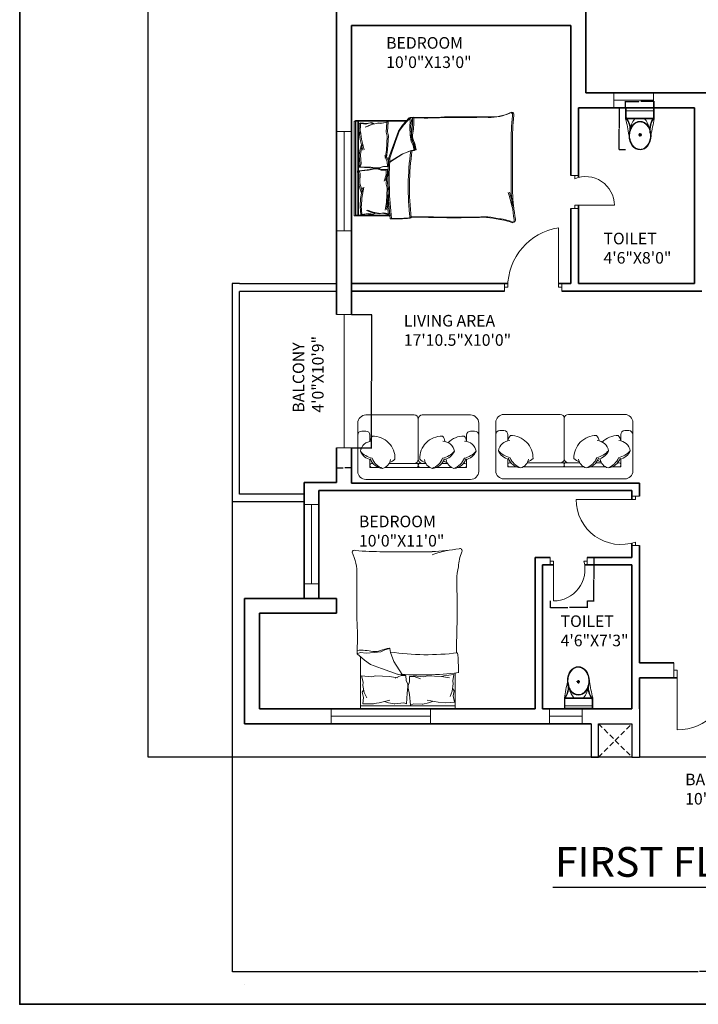
# Model space of a CAD drawing. Units: inches. Extents: x 2296 to 3812, y -1531 to 2564.
# Tile 1 of 10: x 2296 to 2706, y 1124 to 1719. Entities that reach past the tile are written whole.
import ezdxf

# ---------------------------------------------------------------- set-up
doc = ezdxf.new("R2010")
doc.units = ezdxf.units.IN
doc.linetypes.add('HIDDEN2', pattern=[4.7625, 3.175, -1.5875])
for name, color, linetype, lineweight in [('A-ANNO-DIMS', 2, 'Continuous', 18), ('A-ANNO-TEXT', 7, 'Continuous', 25), ('A-ANNO-TTLB', 7, 'Continuous', 35), ('A-AREA-IDEN', 7, 'Continuous', 18), ('A-DOOR', 3, 'Continuous', 18), ('A-FLOR-FIXT', 9, 'Continuous', 18), ('A-FLOR-HRAL', 7, 'Continuous', 25), ('A-FURN', 8, 'Continuous', 18), ('A-GLAZ', 4, 'Continuous', 18), ('A-REF', 8, 'Continuous', 13), ('A-WALL', 7, 'Continuous', 35), ('A-WALL-HIDN', 8, 'HIDDEN2', 18)]:
    doc.layers.add(name, color=color, linetype=linetype, lineweight=lineweight)
doc.styles.get("Standard").update_dxf_attribs({"font": 'arial.ttf'})
doc.dimstyles.get("Standard").update_dxf_attribs({"dimtxt": 0.18, "dimasz": 0.18, "dimexe": 0.18, "dimexo": 0.0625, "dimgap": 0.09, "dimtad": 0, "dimtih": 1, "dimtoh": 1, "dimdec": 4, "dimzin": 0, "dimdsep": 46, "dimtxsty": 'Standard', "dimcen": 0.09, "dimadec": 0, "dimazin": 0, "dimtfac": 1, "dimtdec": 4, "dimtofl": 0, "dimtmove": 0, "dimatfit": 3, "dimfxl": 1, "dimtolj": 1, "dimtzin": 0, "dimarcsym": 0})

# ---------------------------------------------------------------- blocks, each defined once
blk = doc.blocks.new('A$C31115884')
for p, q in [((283, 498), (223, 498)), ((258, 466), (258, 523)), ((0, 200), (0, 0)), ((520, 200), (0, 200)), ((10, 190), (10, 10)), ((510, 190), (10, 190)), ((510, 10), (510, 190)), ((520, 0), (520, 200)), ((510, 54), (0, 54)), ((10, 10), (510, 10)), ((0, 0), (520, 0))]:
    blk.add_line(p, q)
blk.add_circle((256, 496), 23.6)
for centre, radius, start, end in [((2778, -205), 2807, 165.4549, 171.7133), ((-295, 403), 365, 324.2091, 9.3499), ((-295, 403), 375, 324.2091, 9.3499), ((139, 406), 293, 315.8436, 2.6563), ((806, 403), 375, 179.2036, 215.7909), ((806, 403), 365, 170.6501, 215.7909), ((3237, 905), 2807, 188.2867, 194.5451), ((384, 406), 293, 190.2774, 224.1564)]:
    blk.add_arc(centre, radius, start, end)
blk.add_ellipse((256, 510), major_axis=(0, -261), ratio=0.772727)
blk.add_open_spline([(256, 259), (263, 259), (270, 260), (288, 262), (299, 265), (320, 273), (330, 278), (350, 291), (360, 299), (378, 316), (386, 326), (402, 347), (409, 358), (421, 383), (427, 395), (436, 422), (440, 436), (445, 465), (447, 480), (448, 509), (448, 524), (445, 553), (443, 568), (436, 596), (432, 610), (422, 636), (416, 649), (402, 672), (395, 683), (379, 703), (370, 712), (351, 728), (341, 735), (321, 746), (310, 751), (289, 757), (278, 759), (256, 761), (245, 761), (223, 757), (212, 754), (191, 746), (181, 741), (161, 728), (151, 720), (133, 703), (125, 693), (110, 672), (103, 660), (90, 636), (85, 623), (76, 596), (72, 582), (67, 553), (66, 538), (64, 509), (65, 494), (68, 465), (70, 450), (77, 422), (81, 408), (91, 382), (97, 370), (111, 346), (118, 335), (135, 316), (144, 307), (162, 291), (172, 284), (193, 273), (203, 269), (225, 262), (236, 260), (250, 259), (253, 259), (256, 259)], degree=3, knots=[0, 0, 0, 0, 0.110105, 0.110105, 0.285049, 0.285049, 0.459994, 0.459994, 0.634938, 0.634938, 0.809882, 0.809882, 0.984827, 0.984827, 1.159771, 1.159771, 1.334715, 1.334715, 1.50966, 1.50966, 1.684604, 1.684604, 1.859549, 1.859549, 2.034493, 2.034493, 2.209437, 2.209437, 2.384382, 2.384382, 2.559326, 2.559326, 2.73427, 2.73427, 2.909215, 2.909215, 3.084159, 3.084159, 3.259103, 3.259103, 3.434048, 3.434048, 3.608992, 3.608992, 3.783936, 3.783936, 3.958881, 3.958881, 4.133825, 4.133825, 4.30877, 4.30877, 4.483714, 4.483714, 4.658658, 4.658658, 4.833603, 4.833603, 5.008547, 5.008547, 5.183491, 5.183491, 5.358436, 5.358436, 5.53338, 5.53338, 5.708324, 5.708324, 5.883269, 5.883269, 6.058213, 6.058213, 6.233158, 6.233158, 6.283185, 6.283185, 6.283185, 6.283185])
blk = doc.blocks.new('DOOR-BEDROOM-36-WS')
for p, q in [((32.71, 2.25), (32.71, 38.25)), ((0, 4.5), (0, 0)), ((0, 0), (0, 2.25)), ((0, 2.25), (2, 2.25)), ((34.71, 2.25), (32.71, 2.25)), ((34.71, 4.5), (34.71, 0)), ((34.71, 0), (34.71, 2.25))]:
    blk.add_line(p, q)
blk.add_arc((38.45, 2.25), 36.46, 99.06194, 180)
blk = doc.blocks.new('DOOR-BATH-24-SW')
for p, q in [((0, 26.25), (0, 21.75)), ((0, 21.75), (0, 24)), ((0, 24), (2, 24)), ((2, 24), (2, 0)), ((22.44, 24), (20.44, 24)), ((22.44, 26.25), (22.44, 21.75)), ((22.44, 21.75), (22.44, 24))]:
    blk.add_line(p, q)
blk.add_arc((2, 19.08), 19.08, 270, 14.93359)
blk = doc.blocks.new('DOOR-BEDROOM-36-SW')
for p, q in [((36, 27.71), (0, 27.71)), ((38.25, 29.71), (33.75, 29.71)), ((33.75, 29.71), (36, 29.71)), ((36, 29.71), (36, 27.71)), ((36, 0), (36, 2)), ((33.75, 0), (38.25, 0)), ((38.25, 0), (36, 0))]:
    blk.add_line(p, q)
blk.add_arc((27.18, 27.71), 27.18, 180, 288.93127)
blk = doc.blocks.new('DOOR-BALCONY-PAIR-S')
for p, q in [((0, 40.5), (0, 31.5)), ((0, 31.5), (0, 36)), ((0, 36), (2, 36)), ((2, 36), (2, 0)), ((65.68, 36), (63.68, 36)), ((63.68, 36), (63.68, 0)), ((65.68, 40.5), (65.68, 31.5)), ((65.68, 31.5), (65.68, 36))]:
    blk.add_line(p, q)
for centre, radius, start, end in [((2, 31.87), 31.87, 270, 359.32793), ((65.8, 31.86), 31.93, 180.64039, 266.18908)]:
    blk.add_arc(centre, radius, start, end)
blk = doc.blocks.new('DOOR-BATH-24-WS')
for p, q in [((0, 20), (4.5, 20)), ((4.5, 20), (2.25, 20)), ((2.25, 20), (2.25, 18)), ((2.25, 0), (2.25, 2)), ((2.25, 2), (26.25, 2)), ((0, 0), (4.5, 0)), ((4.5, 0), (2.25, 0))]:
    blk.add_line(p, q)
blk.add_arc((8.92, 2), 17.33, 0, 112.62699)
blk = doc.blocks.new('WIN-60-JAMB-A')
for p, q in [((0, 60), (9, 60)), ((9, 60), (4.5, 60)), ((4.5, 60), (4.5, 0)), ((9, 0), (0, 0)), ((4.5, 0), (9, 0))]:
    blk.add_line(p, q)
blk = doc.blocks.new('WIN-48-BEDROOM-SW')
for p, q in [((0, 48), (9, 48)), ((9, 48), (4.5, 48)), ((4.5, 48), (4.5, 0)), ((9, 0), (0, 0)), ((4.5, 0), (9, 0))]:
    blk.add_line(p, q)
blk = doc.blocks.new('WIN-24-SHAFT-S')
for p, q in [((0, 9), (0, 0)), ((24, 4.5), (24, 9)), ((24, 9), (24, 0)), ((0, 0), (0, 4.5)), ((0, 4.5), (0, 4.5)), ((0, 4.5), (24, 4.5))]:
    blk.add_line(p, q)
blk = doc.blocks.new('WIN-60-SILL')
for p, q in [((0, 9), (0, 0)), ((60, 4.5), (60, 9)), ((60, 9), (60, 0)), ((0, 0), (0, 4.5)), ((0, 4.5), (60, 4.5))]:
    blk.add_line(p, q)
blk = doc.blocks.new('WIN-20-VENT')
for p, q in [((0, 9), (0, 0)), ((19.57, 4.5), (19.57, 9)), ((19.57, 9), (19.57, 0)), ((0, 0), (0, 4.5)), ((0, 4.5), (0, 4.5)), ((0, 4.5), (19.57, 4.5)), ((19.57, 0), (19.57, 0))]:
    blk.add_line(p, q)
blk = doc.blocks.new('GLAZ-BALCONY-S')
for p, q in [((0, 80.52), (9, 80.52)), ((4.5, 80.52), (4.5, 0)), ((0, 0), (9, 0))]:
    blk.add_line(p, q)
blk = doc.blocks.new('BED-DOUBLE')
for p, q in [((48.49, 95), (18.98, 95)), ((22.83, 36.42), (19.86, 35.68)), ((23.21, 34.01), (22.83, 36.42)), ((3.07, 35.36), (3.17, 33.26, 4.64)), ((5.01, 34.01), (3.17, 33.26)), ((3.17, 33.26), (7.61, 29.37)), ((8.72, 33.63), (5.01, 34.01)), ((5.09, 0), (5.09, 31.9)), ((13.37, 34.01), (8.72, 33.63)), ((17.45, 34.56), (13.37, 34.01)), ((19.86, 35.68), (17.45, 34.56)), ((25.25, 28.62), (23.21, 34.01)), ((7.61, 29.37), (11.14, 26.77)), ((11.14, 26.77), (17.82, 24.36)), ((17.82, 24.36), (27.82, 20.84)), ((30.27, 20.84), (25.25, 28.62)), ((11.92, 19.38), (5.77, 19.87)), ((5.77, 19.87), (6.7, 16.11)), ((14.27, 20.05), (11.92, 19.38)), ((22.67, 19.54), (14.27, 20.05)), ((27.51, 18.74), (22.67, 19.54)), ((29.68, 20.07), (26, 18.53)), ((32.62, 20.25), (29.68, 20.07)), ((32.82, 17.04), (32.62, 20.25)), ((34.71, 16.28), (34.71, 19.5)), ((34.71, 19.5), (37.65, 19.5)), ((43.31, 19.38), (37.16, 19.87)), ((37.65, 19.5), (41.42, 18.19)), ((45.66, 20.05), (43.31, 19.38)), ((54.06, 19.54), (45.66, 20.05)), ((54.06, 19.54), (55.42, 19.92)), ((58.9, 18.74), (54.06, 19.54)), ((55.42, 19.92), (61.53, 20.79)), ((61.53, 20.79), (60.84, 16.98)), ((62.38, 21.71), (62.38, 0)), ((6.7, 16.11), (6.47, 14.18)), ((6.47, 14.18), (7.43, 9.9)), ((33.66, 14.84), (32.82, 17.04)), ((33.3, 9.43), (33.75, 13.28)), ((33.75, 13.28), (33.66, 14.84)), ((34.01, 14.03), (34.71, 16.28)), ((34.01, 12.47), (34.01, 14.03)), ((34.71, 8.66), (34.01, 12.47)), ((61.19, 15.07), (60.49, 10.74)), ((60.84, 16.98), (61.19, 15.07)), ((61.71, 10.91), (61.01, 12.12)), ((6.21, 10), (6.83, 11.25)), ((6.93, 6.92), (6.21, 10)), ((6.47, 3.07), (6.93, 6.92)), ((7.43, 9.9), (8.85, 6.69)), ((33.01, 2.99), (33.3, 9.43)), ((35.4, 2.24), (34.71, 8.66)), ((60.49, 10.74), (59.28, 7.44)), ((61.19, 7.79), (61.71, 10.91)), ((61.88, 3.98), (61.19, 7.79)), ((62.38, 1.84), (5.09, 1.84)), ((62.38, 0), (5.09, 0)), ((6.47, 3.07), (12.95, 2.95)), ((11.75, 3.05), (16.3, 3.68)), ((12.95, 2.95), (11.75, 3.05)), ((16.3, 3.68), (22.8, 5.3)), ((19.55, 4.4), (22.03, 3.69)), ((22.03, 3.69), (25.54, 3.04)), ((25.54, 3.04), (25.93, 3.07)), ((25.93, 3.07), (31.24, 3.57)), ((31.24, 3.57), (33.01, 2.99)), ((37.13, 2.94), (35.4, 2.24)), ((42.46, 2.76), (37.13, 2.94)), ((42.85, 2.76), (42.46, 2.76)), ((46.31, 3.63), (42.85, 2.76)), ((52.03, 3.98), (45.45, 5.19)), ((48.74, 4.5), (46.31, 3.63)), ((56.62, 3.63), (52.03, 3.98)), ((56.74, 3.61), (56.62, 3.63)), ((61.87, 4), (56.74, 3.61))]:
    blk.add_line(p, q)
for centre, radius, start, end in [((1.32, 94.55), 1.32, 62.65876, 176.02002), ((17.21, 254.49), 159.5, 264.4998, 270.63509), ((87.19, -28.43), 127.63, 103.38322, 107.70533), ((40.86, 240.78), 145.97, 272.99578, 279.40907), ((65.24, 95.57), 1.31, 326.17358, 113.47814), ((-24.75, 82.32), 27.65, 357.47136, 26.46809), ((92.52, 84.25), 28.25, 157.97508, 176.652), ((98.8, 77.34), 35.53, 166.06484, 178.91125), ((5471.89, 81.31), 5469.02, 180.00217, 180.28689), ((-514.68, 60.68), 578.22, 358.22771, 1.71854), ((-151.96, 43.54), 155.25, 356.97912, 3.83645), ((267.13, 37.37), 203.94, 178.4762, 181.00819), ((29.2, 1.78), 35.55, 100.66171, 109.88058), ((22.63, 36.49), 0.221, 340.24637, 91.13765), ((5.01, -7.98), 43.38, 79.87628, 92.56571), ((14.11, 42.04), 7.46, 258.6608, 293.73842), ((45.26, 187.4), 154.68, 261.78449, 276.90062), ((-35.55, 24.09), 99.87, 358.72178, 5.60397), ((40.94, 218.26), 197.77, 266.08655, 276.78213)]:
    blk.add_arc(centre, radius, start, end)
blk = doc.blocks.new('*D45')
at = {"layer": 'A-ANNO-DIMS', "color": 0, "lineweight": -2, "transparency": 16777216}
for p, q in [((2662.39, 1665.95), (2658.45, 1665.95)), ((2658.63, 1665.77), (2658.63, 1653.39)), ((2658.63, 1640.65), (2658.63, 1653.03)), ((2662.39, 1640.47), (2658.45, 1640.47))]:
    blk.add_line(p, q, dxfattribs=at)
at = {"layer": 'A-ANNO-DIMS', "color": 0, "transparency": 16777216}
for points in [[(2658.6, 1665.77), (2658.66, 1665.77), (2658.63, 1665.95)], [(2658.6, 1640.65), (2658.66, 1640.65), (2658.63, 1640.47)]]:
    blk.add_solid(points, dxfattribs=at)
at = {"layer": 'Defpoints', "color": 0, "transparency": 16777216}
for p in [(2662.45, 1665.95), (2658.63, 1640.47), (2662.45, 1640.47)]:
    blk.add_point(p, dxfattribs=at)
at = {"layer": 'A-ANNO-DIMS', "color": 0, "transparency": 16777216, "insert": (2658.63, 1653.21), "char_height": 0.18, "attachment_point": 5}
blk.add_mtext('\\A1;WC 25 TYP.', dxfattribs=at)
blk = doc.blocks.new('*D46')
at = {"layer": 'A-ANNO-DIMS', "color": 0, "lineweight": -2, "transparency": 16777216}
for p, q in [((2662.45, 1666.01), (2662.45, 1669.95)), ((2662.63, 1669.77), (2670.53, 1669.77)), ((2679.46, 1669.77), (2671.57, 1669.77)), ((2679.64, 1666.01), (2679.64, 1669.95))]:
    blk.add_line(p, q, dxfattribs=at)
at = {"layer": 'A-ANNO-DIMS', "color": 0, "transparency": 16777216}
for points in [[(2662.63, 1669.8), (2662.63, 1669.74), (2662.45, 1669.77)], [(2679.46, 1669.8), (2679.46, 1669.74), (2679.64, 1669.77)]]:
    blk.add_solid(points, dxfattribs=at)
at = {"layer": 'Defpoints', "color": 0, "transparency": 16777216}
for p in [(2662.45, 1669.77), (2662.45, 1665.95), (2679.64, 1665.95)]:
    blk.add_point(p, dxfattribs=at)
at = {"layer": 'A-ANNO-DIMS', "color": 0, "transparency": 16777216, "insert": (2671.05, 1669.77), "char_height": 0.18, "attachment_point": 5}
blk.add_mtext('\\A1;17 TYP.', dxfattribs=at)
blk = doc.blocks.new('*D83')
at = {"layer": 'A-ANNO-DIMS', "color": 0, "lineweight": -2, "transparency": 16777216}
for p, q in [((2639.31, 1394.1), (2643.37, 1394.1)), ((2643.19, 1393.92), (2643.19, 1381.16)), ((2643.19, 1368.03), (2643.19, 1380.79)), ((2639.31, 1367.85), (2643.37, 1367.85))]:
    blk.add_line(p, q, dxfattribs=at)
at = {"layer": 'A-ANNO-DIMS', "color": 0, "transparency": 16777216}
for points in [[(2643.16, 1393.92), (2643.22, 1393.92), (2643.19, 1394.1)], [(2643.16, 1368.03), (2643.22, 1368.03), (2643.19, 1367.85)]]:
    blk.add_solid(points, dxfattribs=at)
at = {"layer": 'Defpoints', "color": 0, "transparency": 16777216}
for p in [(2639.25, 1394.1), (2643.19, 1394.1), (2639.25, 1367.85)]:
    blk.add_point(p, dxfattribs=at)
at = {"layer": 'A-ANNO-DIMS', "color": 0, "transparency": 16777216, "insert": (2643.19, 1380.98), "char_height": 0.18, "attachment_point": 5}
blk.add_mtext('\\A1;BATH DOOR 26 TYP.', dxfattribs=at)
blk = doc.blocks.new('*D84')
at = {"layer": 'A-ANNO-DIMS', "color": 0, "lineweight": -2, "transparency": 16777216}
for p, q in [((2616.81, 1367.79), (2616.81, 1363.73)), ((2616.99, 1363.91), (2627.5, 1363.91)), ((2639.07, 1363.91), (2628.56, 1363.91)), ((2639.25, 1367.79), (2639.25, 1363.73))]:
    blk.add_line(p, q, dxfattribs=at)
at = {"layer": 'A-ANNO-DIMS', "color": 0, "transparency": 16777216}
for points in [[(2616.99, 1363.94), (2616.99, 1363.88), (2616.81, 1363.91)], [(2639.07, 1363.94), (2639.07, 1363.88), (2639.25, 1363.91)]]:
    blk.add_solid(points, dxfattribs=at)
at = {"layer": 'Defpoints', "color": 0, "transparency": 16777216}
for p in [(2616.81, 1367.85), (2639.25, 1367.85), (2639.25, 1363.91)]:
    blk.add_point(p, dxfattribs=at)
at = {"layer": 'A-ANNO-DIMS', "color": 0, "transparency": 16777216, "insert": (2628.03, 1363.91), "char_height": 0.18, "attachment_point": 5}
blk.add_mtext('\\A1;22 TYP.', dxfattribs=at)
blk = doc.blocks.new('*D123')
at = {"layer": 'A-ANNO-DIMS', "color": 0, "lineweight": -2, "transparency": 16777216}
for p, q in [((2496.81, 1540.93), (2509.01, 1540.93)), ((2508.83, 1540.75), (2508.83, 1500.85)), ((2508.83, 1460.59), (2508.83, 1500.49)), ((2496.81, 1460.41), (2509.01, 1460.41))]:
    blk.add_line(p, q, dxfattribs=at)
at = {"layer": 'A-ANNO-DIMS', "color": 0, "transparency": 16777216}
for points in [[(2508.8, 1540.75), (2508.86, 1540.75), (2508.83, 1540.93)], [(2508.8, 1460.59), (2508.86, 1460.59), (2508.83, 1460.41)]]:
    blk.add_solid(points, dxfattribs=at)
at = {"layer": 'Defpoints', "color": 0, "transparency": 16777216}
for p in [(2496.75, 1540.93), (2508.83, 1540.93), (2496.75, 1460.41)]:
    blk.add_point(p, dxfattribs=at)
at = {"layer": 'A-ANNO-DIMS', "color": 0, "transparency": 16777216, "insert": (2508.83, 1500.67), "char_height": 0.18, "attachment_point": 5}
blk.add_mtext('\\A1;GLAZING 81 TYP.', dxfattribs=at)
blk = doc.blocks.new('*D124')
at = {"layer": 'A-ANNO-DIMS', "color": 0, "lineweight": -2, "transparency": 16777216}
for p, q in [((2487.75, 1460.35), (2487.75, 1448.15)), ((2496.75, 1460.35), (2496.75, 1448.15)), ((2487.93, 1448.33), (2491.79, 1448.33)), ((2496.57, 1448.33), (2492.71, 1448.33))]:
    blk.add_line(p, q, dxfattribs=at)
at = {"layer": 'A-ANNO-DIMS', "color": 0, "transparency": 16777216}
for points in [[(2487.93, 1448.36), (2487.93, 1448.3), (2487.75, 1448.33)], [(2496.57, 1448.36), (2496.57, 1448.3), (2496.75, 1448.33)]]:
    blk.add_solid(points, dxfattribs=at)
at = {"layer": 'Defpoints', "color": 0, "transparency": 16777216}
for p in [(2487.75, 1460.41), (2496.75, 1460.41), (2496.75, 1448.33)]:
    blk.add_point(p, dxfattribs=at)
at = {"layer": 'A-ANNO-DIMS', "color": 0, "transparency": 16777216, "insert": (2492.25, 1448.33), "char_height": 0.18, "attachment_point": 5}
blk.add_mtext('\\A1;9 TYP.', dxfattribs=at)
blk = doc.blocks.new('*D127')
at = {"layer": 'A-ANNO-DIMS', "color": 0, "lineweight": -2, "transparency": 16777216}
for p, q in [((2988.9, 1498.34), (2988.9, 1143.72)), ((2424.57, 1427.77), (2424.57, 1143.72)), ((2424.75, 1143.9), (2706.34, 1143.9)), ((2988.72, 1143.9), (2707.13, 1143.9))]:
    blk.add_line(p, q, dxfattribs=at)
at = {"layer": 'A-ANNO-DIMS', "color": 0, "transparency": 16777216}
for points in [[(2424.75, 1143.93), (2424.75, 1143.87), (2424.57, 1143.9)], [(2988.72, 1143.93), (2988.72, 1143.87), (2988.9, 1143.9)]]:
    blk.add_solid(points, dxfattribs=at)
at = {"layer": 'Defpoints', "color": 0, "transparency": 16777216}
for p in [(2988.9, 1498.4), (2424.57, 1427.84), (2988.9, 1143.9)]:
    blk.add_point(p, dxfattribs=at)
at = {"layer": 'A-ANNO-DIMS', "color": 0, "transparency": 16777216, "insert": (2706.74, 1143.9), "char_height": 0.18, "attachment_point": 5}
blk.add_mtext('\\A1;564.3', dxfattribs=at)
blk = doc.blocks.new('*D128')
at = {"layer": 'A-ANNO-DIMS', "color": 0, "lineweight": -2, "transparency": 16777216}
for p, q in [((2660.01, 2175.03), (2373.54, 2175.03)), ((2373.72, 2174.85), (2373.72, 1724.41)), ((2373.72, 1273.61), (2373.72, 1724.05)), ((2666.19, 1273.43), (2373.54, 1273.43))]:
    blk.add_line(p, q, dxfattribs=at)
at = {"layer": 'A-ANNO-DIMS', "color": 0, "transparency": 16777216}
for points in [[(2373.69, 2174.85), (2373.75, 2174.85), (2373.72, 2175.03)], [(2373.69, 1273.61), (2373.75, 1273.61), (2373.72, 1273.43)]]:
    blk.add_solid(points, dxfattribs=at)
at = {"layer": 'Defpoints', "color": 0, "transparency": 16777216}
for p in [(2373.72, 2175.03), (2660.07, 2175.03), (2666.25, 1273.43)]:
    blk.add_point(p, dxfattribs=at)
at = {"layer": 'A-ANNO-DIMS', "color": 0, "transparency": 16777216, "insert": (2373.72, 1724.23), "char_height": 0.18, "attachment_point": 5}
blk.add_mtext('\\A1;901.6', dxfattribs=at)

msp = doc.modelspace()

# ---------------------------------------------------------------- linework, layer by layer
at = {"layer": 'A-ANNO-TEXT'}
msp.add_line((2618.3678, 1194.7471), (2857.1248, 1194.7471), dxfattribs=at)
at = {"layer": 'A-ANNO-TTLB'}
msp.add_lwpolyline([(2296.1257, 2564.2989), (3812.4193, 2564.2989), (3812.4193, 1124.0028), (2296.1257, 1124.0028)], close=True, dxfattribs=at)
at = {"layer": 'A-FLOR-HRAL'}
for p, q in [((2424.5693, 1559.6578), (2424.5693, 1427.8367)), ((2429.0693, 1559.6578), (2424.5693, 1559.6578)), ((2429.0693, 1559.6578), (2487.7523, 1559.6578)), ((2429.0693, 1432.3367), (2429.0693, 1554.9294)), ((2487.7523, 1554.9294), (2429.0693, 1554.9294)), ((2468.0693, 1431.0117), (2468.0693, 1435.5117)), ((2468.0693, 1432.3367), (2429.0693, 1432.3367)), ((2468.0693, 1427.8367), (2468.0693, 1432.3367)), ((2424.5693, 1427.8367), (2468.0693, 1427.8367)), ((2670.7523, 1302.6012), (2670.7523, 1273.434)), ((2641.5757, 1293.6012), (2641.5757, 1273.434)), ((2646.0757, 1273.434), (2646.0757, 1293.6012)), ((2646.0757, 1293.6012), (2666.2523, 1293.6012)), ((2666.2523, 1293.6012), (2666.2523, 1273.434)), ((2641.5757, 1273.434), (2646.0757, 1273.434)), ((2666.2523, 1273.434), (2670.7523, 1273.434)), ((2784.5693, 1273.434), (2670.7523, 1273.434))]:
    msp.add_line(p, q, dxfattribs=at)
at = {"layer": 'A-FURN', "ltscale": 0.03}
for points in [[(2534.6414, 1480.2223, -0.41421356), (2537.0777, 1477.786, -0.41421356), (2539.514, 1480.2223), (2568.7498, 1480.2223, -0.41421356), (2573.6224, 1475.3497), (2573.6224, 1446.1139, -0.41421356), (2568.7498, 1441.2413), (2505.4056, 1441.2413, -0.41421356), (2500.5329, 1446.1139), (2500.5329, 1475.3497, -0.41421356), (2505.4056, 1480.2223), (2534.6414, 1480.2223, -0.41421356), (2537.0777, 1477.786, -0.41421356), (2539.514, 1480.2223)], [(2622.9591, 1480.5496, -0.41421356), (2625.3954, 1478.1133, -0.41421356), (2627.8317, 1480.5496), (2661.9401, 1480.5496, -0.41421356), (2666.8128, 1475.677), (2666.8128, 1446.4412, -0.41421356), (2661.9401, 1441.5686), (2588.8507, 1441.5686, -0.41421356), (2583.978, 1446.4412), (2583.978, 1475.677, -0.41421356), (2588.8507, 1480.5496), (2622.9591, 1480.5496, -0.41421356), (2625.3954, 1478.1133, -0.41421356), (2627.8317, 1480.5496)]]:
    msp.add_lwpolyline(points, format="xyb", dxfattribs=at)
at = {"layer": 'A-FURN'}
for points in [[(2534.6414, 1450.9865, 0.41421356), (2537.0777, 1453.4228), (2537.0777, 1477.786, 0.41421356)], [(2539.514, 1450.9865, -0.41421356), (2537.0777, 1453.4228), (2537.0777, 1477.786, -0.41421356)], [(2622.9591, 1451.3138, 0.41421356), (2625.3954, 1453.7501), (2625.3954, 1478.1133, 0.41421356)], [(2627.8317, 1451.3138, -0.41421356), (2625.3954, 1453.7501), (2625.3954, 1478.1133, -0.41421356)], [(2500.5329, 1468.0407, -0.41421356), (2502.9693, 1470.477), (2505.4056, 1470.477, -0.41421356), (2507.8419, 1468.0407), (2507.8419, 1464.266)], [(2566.3135, 1464.266), (2566.3135, 1468.0407, -0.41421356), (2568.7498, 1470.477), (2571.1861, 1470.477, -0.41421356), (2573.6224, 1468.0407)], [(2583.978, 1468.368, -0.41421356), (2586.4143, 1470.8044), (2588.8507, 1470.8044, -0.41421356), (2591.287, 1468.368), (2591.287, 1464.5933)], [(2659.5038, 1464.5933), (2659.5038, 1468.368, -0.41421356), (2661.9401, 1470.8044), (2664.3765, 1470.8044, -0.41421356), (2666.8128, 1468.368)], [(2509.0645, 1464.4134, 0.35677236), (2502.0835, 1458.2724, 0.24954205), (2508.409, 1453.2117, -9.61688035)], [(2507.8366, 1464.2649, -0.16554063), (2509.3438, 1467.4839, -0.42598917), (2523.0266, 1453.5271, -0.12152332), (2519.7786, 1451.6034, 7.11546429)], [(2553.1944, 1464.2649, 0.16554063), (2551.6873, 1467.4839, 0.42598917), (2538.0044, 1453.5271, 0.12152332), (2541.2525, 1451.6034, -7.11546429)], [(2551.9665, 1464.4134, -0.35677236), (2558.9475, 1458.2724, -0.24954205), (2552.6221, 1453.2117, 9.61688035)], [(2566.3188, 1464.2649, 0.16554063), (2564.8116, 1467.4839, 0.20023115), (2555.1403, 1463.5634, 0.12152332)], [(2565.0908, 1464.4134, -0.35677236), (2572.0719, 1458.2724, -0.24954205), (2565.7464, 1453.2117, 9.61688035)], [(2592.5096, 1464.7407, 0.35677236), (2585.5286, 1458.5997, 0.24954205), (2591.854, 1453.539, -9.61688035)], [(2591.2817, 1464.5922, -0.16554063), (2592.7889, 1467.8113, -0.42598917), (2606.4717, 1453.8544, -0.12152332), (2603.2236, 1451.9307, 7.11546429)], [(2646.3848, 1464.5922, 0.16554063), (2644.8776, 1467.8113, 0.42598917), (2631.1948, 1453.8544, 0.12152332), (2634.4428, 1451.9307, -7.11546429)], [(2645.1568, 1464.7407, -0.35677236), (2652.1379, 1458.5997, -0.24954205), (2645.8124, 1453.539, 9.61688035)], [(2659.5091, 1464.5922, 0.16554063), (2658.0019, 1467.8113, 0.20023115), (2648.3307, 1463.8908, 0.12152332)], [(2658.2812, 1464.7407, -0.35677236), (2665.2622, 1458.5997, -0.24954205), (2658.9368, 1453.539, 9.61688035)], [(2502.0835, 1458.2724, 0.14772988), (2509.2042, 1454.0854, 0.21334276), (2515.4871, 1447.9444, 0.17866181)], [(2558.9475, 1458.2724, -0.14772988), (2551.8269, 1454.0854, -0.21334276), (2545.544, 1447.9444, -0.17866181)], [(2572.0719, 1458.2724, -0.14772988), (2564.9512, 1454.0854, -0.21334276), (2558.6683, 1447.9444, -0.17866181)], [(2585.5286, 1458.5997, 0.14772988), (2592.6492, 1454.4127, 0.21334276), (2598.9322, 1448.2717, 0.17866181)], [(2652.1379, 1458.5997, -0.14772988), (2645.0172, 1454.4127, -0.21334276), (2638.7343, 1448.2717, -0.17866181)], [(2665.2622, 1458.5997, -0.14772988), (2658.1416, 1454.4127, -0.21334276), (2651.8586, 1448.2717, -0.17866181)], [(2508.2204, 1453.7517, 0.30666349), (2515.4871, 1447.9444, 0.30632997), (2520.2342, 1453.248, -0.87284716)], [(2534.6414, 1450.9865, 0.41421356), (2537.0777, 1453.4228)], [(2539.514, 1450.9865, -0.41421356), (2537.0777, 1453.4228)], [(2552.8106, 1453.7517, -0.30666349), (2545.544, 1447.9444, -0.30632997), (2540.7968, 1453.248, 0.87284716)], [(2552.3342, 1452.5559, 0.07186538), (2554.3768, 1451.6034, -7.11546429)], [(2565.9349, 1453.7517, -0.30666349), (2558.6683, 1447.9444, -0.30632997), (2553.9212, 1453.248, 0.87284716)], [(2561.1881, 1448.5502), (2566.3135, 1448.5502), (2566.3135, 1453.3381, -0.41421356)], [(2591.6655, 1454.079, 0.30666349), (2598.9322, 1448.2717, 0.30632997), (2603.6793, 1453.5753, -0.87284716)], [(2622.9591, 1451.3138, 0.41421356), (2625.3954, 1453.7501)], [(2627.8317, 1451.3138, -0.41421356), (2625.3954, 1453.7501)], [(2646.0009, 1454.079, -0.30666349), (2638.7343, 1448.2717, -0.30632997), (2633.9872, 1453.5753, 0.87284716)], [(2645.5246, 1452.8832, 0.07186538), (2647.5672, 1451.9307, -7.11546429)], [(2659.1253, 1454.079, -0.30666349), (2651.8586, 1448.2717, -0.30632997), (2647.1115, 1453.5753, 0.87284716)], [(2654.3785, 1448.8775), (2659.5038, 1448.8775), (2659.5038, 1453.6655, -0.41421356)], [(2509.7011, 1450.9865), (2508.8164, 1450.9865, 0.41421356), (2507.8419, 1450.012), (2507.8419, 1449.5247, 0.41421356), (2508.8164, 1448.5502)], [(2508.8164, 1448.5502), (2512.9672, 1448.5502, 0.41421356)], [(2517.0204, 1448.5502), (2536.1032, 1448.5502, 0.41421356), (2537.0777, 1449.5247), (2537.0777, 1450.012, 0.41421356), (2536.1032, 1450.9865), (2519.4736, 1450.9865, 0.41421356)], [(2544.0107, 1448.5502), (2538.0522, 1448.5502, -0.41421356), (2537.0777, 1449.5247), (2537.0777, 1450.012, -0.41421356), (2538.0522, 1450.9865), (2541.5574, 1450.9865, -0.41421356)], [(2557.135, 1448.5502), (2548.0638, 1448.5502, -0.41421356)], [(2551.3299, 1450.9865), (2554.6818, 1450.9865, -0.41421356)], [(2565.339, 1448.5502), (2561.1881, 1448.5502, -0.41421356)], [(2564.4543, 1450.9865), (2565.339, 1450.9865, -0.41421356), (2566.3135, 1450.012), (2566.3135, 1449.5247, -0.41421356), (2565.339, 1448.5502)], [(2593.1462, 1451.3138), (2592.2615, 1451.3138, 0.41421356), (2591.287, 1450.3393), (2591.287, 1449.852, 0.41421356), (2592.2615, 1448.8775)], [(2592.2615, 1448.8775), (2596.4123, 1448.8775, 0.41421356)], [(2600.4655, 1448.8775), (2624.4209, 1448.8775, 0.41421356), (2625.3954, 1449.852), (2625.3954, 1450.3393, 0.41421356), (2624.4209, 1451.3138), (2602.9187, 1451.3138, 0.41421356)], [(2637.201, 1448.8775), (2626.3699, 1448.8775, -0.41421356), (2625.3954, 1449.852), (2625.3954, 1450.3393, -0.41421356), (2626.3699, 1451.3138), (2634.7478, 1451.3138, -0.41421356)], [(2650.3253, 1448.8775), (2641.2542, 1448.8775, -0.41421356)], [(2644.5203, 1451.3138), (2647.8721, 1451.3138, -0.41421356)], [(2658.5293, 1448.8775), (2654.3785, 1448.8775, -0.41421356)], [(2657.6446, 1451.3138), (2658.5293, 1451.3138, -0.41421356), (2659.5038, 1450.3393), (2659.5038, 1449.852, -0.41421356), (2658.5293, 1448.8775)]]:
    msp.add_lwpolyline(points, format="xyb", dxfattribs=at)
for points in [[(2507.8419, 1453.3381), (2507.8419, 1448.5502), (2512.9672, 1448.5502)], [(2591.287, 1453.6655), (2591.287, 1448.8775), (2596.4123, 1448.8775)], [(2517.0204, 1448.5502), (2544.0107, 1448.5502)], [(2548.0638, 1448.5502), (2557.135, 1448.5502)], [(2600.4655, 1448.8775), (2637.201, 1448.8775)], [(2641.2542, 1448.8775), (2650.3253, 1448.8775)]]:
    msp.add_lwpolyline(points, dxfattribs=at)
for points in [[(2536.1032, 1448.5502), (2538.0522, 1448.5502, -0.41421356), (2537.0777, 1449.5247), (2537.0777, 1450.012, -0.41421356), (2538.0522, 1450.9865), (2536.1032, 1450.9865, -0.41421356), (2537.0777, 1450.012), (2537.0777, 1449.5247, -0.41421356)], [(2624.4209, 1448.8775), (2626.3699, 1448.8775, -0.41421356), (2625.3954, 1449.852), (2625.3954, 1450.3393, -0.41421356), (2626.3699, 1451.3138), (2624.4209, 1451.3138, -0.41421356), (2625.3954, 1450.3393), (2625.3954, 1449.852, -0.41421356)]]:
    msp.add_lwpolyline(points, format="xyb", close=True, dxfattribs=at)
at = {"layer": 'A-REF'}
msp.add_line((2432.0693, 1136.0111), (2432.0693, 1136.0111), dxfattribs=at)
at = {"layer": 'A-WALL'}
for p, q in [((2487.7523, 1901.6355), (2487.7523, 1540.9318)), ((2638.4, 1780.1578), (2638.4, 1715.6578)), ((2496.7523, 1715.6578), (2614.217, 1715.6578)), ((2496.7523, 1715.6578), (2496.7523, 1555.1578)), ((2614.217, 1715.6578), (2629.4, 1715.6578)), ((2629.4, 1715.6578), (2629.4, 1624.9927)), ((2638.4, 1715.6578), (2638.4, 1674.9485)), ((2638.4, 1674.9485), (2713.1754, 1674.9485)), ((2704.1754, 1665.9485), (2633.9, 1665.9485)), ((2633.9, 1623.7542), (2633.9, 1665.9485)), ((2704.1754, 1665.9485), (2704.1754, 1599.9948)), ((2633.9, 1559.6578), (2633.9, 1606.9949)), ((2629.4, 1604.9949), (2629.4, 1559.6578)), ((2704.1754, 1599.9948), (2704.1754, 1559.6578)), ((2496.7523, 1559.6578), (2591.2334, 1559.6578)), ((2629.4, 1559.6578), (2621.8772, 1559.6578)), ((2704.1754, 1559.6578), (2633.9, 1559.6578)), ((2496.7523, 1555.1578), (2589.1639, 1555.1578)), ((2496.7523, 1555.1578), (2496.7523, 1540.9318)), ((2623.8772, 1555.1578), (2629.4, 1555.1578)), ((2629.4, 1555.1578), (2633.9, 1555.1578)), ((2708.6222, 1555.1578), (2633.9, 1555.1578)), ((2487.7523, 1460.4105), (2487.7523, 1439.3482)), ((2496.7523, 1460.4105), (2496.7523, 1439.1012)), ((2468.0693, 1439.3482), (2468.0693, 1434.6012)), ((2487.7523, 1439.3482), (2468.0693, 1439.3482)), ((2468.0693, 1434.6012), (2468.0693, 1369.3709)), ((2477.0693, 1434.6012), (2487.7523, 1434.6012)), ((2487.7523, 1434.6012), (2477.0693, 1434.6012)), ((2477.0693, 1434.6012), (2477.0693, 1369.3709)), ((2487.7523, 1434.6012), (2607.7523, 1434.6012)), ((2612.2523, 1439.1012), (2496.7523, 1439.1012)), ((2612.2523, 1434.6012), (2607.7523, 1434.6012)), ((2612.2523, 1439.1012), (2670.7523, 1439.1012)), ((2666.2523, 1434.6012), (2612.2523, 1434.6012)), ((2666.2523, 1429.1229), (2666.2523, 1434.6012)), ((2670.7523, 1439.1012), (2670.7523, 1434.6012)), ((2670.7523, 1434.6012), (2670.7523, 1431.1229)), ((2666.2523, 1394.1012), (2666.2523, 1402.747)), ((2670.7523, 1401.4117), (2670.7523, 1394.1012)), ((2607.7523, 1394.1012), (2607.7523, 1302.6012)), ((2616.8144, 1394.1012), (2607.7523, 1394.1012)), ((2666.2523, 1394.1012), (2639.2523, 1394.1012)), ((2670.7523, 1389.6012), (2670.7523, 1394.1012)), ((2670.7523, 1330.434), (2670.7523, 1394.1012)), ((2612.2523, 1302.6012), (2612.2523, 1389.6012)), ((2618.8144, 1389.6012), (2612.2523, 1389.6012)), ((2666.2523, 1389.6012), (2637.7095, 1389.6012)), ((2666.2523, 1302.6012), (2666.2523, 1389.6012)), ((2670.7523, 1330.434), (2670.7523, 1389.6012)), ((2432.0693, 1369.3709), (2432.0693, 1293.6012)), ((2487.7523, 1369.3709), (2432.0693, 1369.3709)), ((2487.7523, 1360.3709), (2487.7523, 1369.3709)), ((2441.0693, 1302.6012), (2441.0693, 1360.3709)), ((2441.0693, 1360.3709), (2487.7523, 1360.3709)), ((2691.6251, 1330.434), (2670.7523, 1330.434)), ((2670.7523, 1302.6012), (2670.7523, 1321.434)), ((2670.7523, 1302.6012), (2670.7523, 1321.434)), ((2670.7523, 1321.434), (2693.6251, 1321.434)), ((2441.0693, 1302.6012), (2607.7523, 1302.6012)), ((2441.0693, 1302.6012), (2607.7523, 1302.6012)), ((2612.2523, 1302.6012), (2666.2523, 1302.6012)), ((2612.2523, 1302.6012), (2666.2523, 1302.6012)), ((2432.0693, 1293.6012), (2641.5757, 1293.6012))]:
    msp.add_line(p, q, dxfattribs=at)
at = {"layer": 'A-WALL-HIDN'}
for p, q in [((2646.0757, 1273.434), (2666.2523, 1293.6012)), ((2646.0757, 1293.6012), (2666.2523, 1273.434))]:
    msp.add_line(p, q, dxfattribs=at)

# ---------------------------------------------------------------- block references
at = {"layer": 'A-DOOR'}
for name, p in [('DOOR-BATH-24-WS', (2629.4, 1604.995)), ('DOOR-BEDROOM-36-WS', (2589.164, 1555.158)), ('DOOR-BEDROOM-36-SW', (2632.502, 1401.412)), ('DOOR-BATH-24-SW', (2616.814, 1367.851)), ('DOOR-BALCONY-PAIR-S', (2691.625, 1289.934))]:
    msp.add_blockref(name, p, dxfattribs=at)
at = {"layer": 'A-FLOR-FIXT', "xscale": 0.0330640103915726, "yscale": 0.0330640103915726, "zscale": 0.0330640103915726, "rotation": 180}
msp.add_blockref('A$C31115884', (2679.6447, 1665.9485), dxfattribs=at)
at = {"layer": 'A-FLOR-FIXT', "xscale": 0.0330640103915726, "yscale": 0.0330640103915726, "zscale": 0.0330640103915726}
msp.add_blockref('A$C31115884', (2625.4199, 1302.6012), dxfattribs=at)
at = {"layer": 'A-FURN', "rotation": 270}
for p in [(2498.2859, 1663.0187), (2499.0523, 1663.2925)]:
    msp.add_blockref('BED-DOUBLE', p, dxfattribs=at)
at = {"layer": 'A-FURN'}
msp.add_blockref('BED-DOUBLE', (2497.056, 1302.601), dxfattribs=at)
at = {"layer": 'A-GLAZ'}
for name, p in [('WIN-24-SHAFT-S', (2655.384, 1665.948)), ('GLAZ-BALCONY-S', (2487.752, 1460.411)), ('WIN-48-BEDROOM-SW', (2468.069, 1378.167)), ('WIN-60-SILL', (2484.5336, 1293.601)), ('WIN-20-VENT', (2616.53, 1293.601))]:
    msp.add_blockref(name, p, dxfattribs=at)
at = {"layer": 'A-GLAZ', "rotation": 180}
msp.add_blockref('WIN-60-JAMB-A', (2496.7526, 1651.6229), dxfattribs=at)

# ---------------------------------------------------------------- texts
at = {"layer": 'A-ANNO-TEXT', "insert": (2619.7605, 1219.0643), "char_height": 18, "attachment_point": 1}
msp.add_mtext_dynamic_manual_height_columns('FIRST FLOOR PLAN', width=376.570462, gutter_width=12.5, heights=[0], dxfattribs=at)
at = {"layer": 'A-AREA-IDEN', "char_height": 7, "attachment_point": 1}
for s, width, insert in [('BEDROOM\\P10\'0"X13\'0"', 63.700324, (2517.6973, 1708.6411)), ('TOILET\\P4\'6"X8\'0"', 46.257588, (2649.0827, 1590.3845)), ('LIVING AREA\\P17\'10.5"X10\'0"', 106.896616, (2528.3487, 1540.7099)), ('BEDROOM\\P10\'0"X11\'0"', 142.655962, (2501.2302, 1419.3717)), ('TOILET\\P4\'6"X7\'3"', 63.914357, (2623.1591, 1359.0873)), ('BALCONY\\P10\'4.5"X4\'0"', 89.884194, (2698.4627, 1263.4036))]:
    msp.add_mtext_dynamic_manual_height_columns(s, width=width, gutter_width=12.5, heights=[0], dxfattribs=dict(at, insert=insert))
at = {"layer": 'A-AREA-IDEN', "insert": (2461.1961, 1481.6453), "char_height": 7, "attachment_point": 1, "rotation": 90}
msp.add_mtext_dynamic_manual_height_columns('BALCONY\\P4\'0"X10\'9"', width=115.468243, gutter_width=12.5, heights=[0], dxfattribs=at)

# ---------------------------------------------------------------- dimensions: what is measured, and where the dimension line sits
at = {"layer": 'A-ANNO-DIMS'}
dim = msp.add_linear_dim(base=(2373.7193, 2175.0276), p1=(2666.2523, 1273.434), p2=(2660.0693, 2175.0276), angle=90, dimstyle='Standard', override={"dimdec": 1, "dimlfac": 1, "dimrnd": 0, "dimzin": 0, "dimdsep": 46, "dimlunit": 2}, dxfattribs=at)
dim.commit()
dim.dimension.update_dxf_attribs({"geometry": '*D128', "text_midpoint": (2373.7193, 1724.2308)})
for base, p1, p2, angle, text, picture, middle in [((2662.4514, 1669.7702), (2679.6447, 1665.9485), (2662.4514, 1665.9485), 180, '<> TYP.', '*D46', (2671.048, 1669.7702)), ((2658.6296, 1640.4704), (2662.4514, 1665.9485), (2662.4514, 1640.4704), 270, 'WC <> TYP.', '*D45', (2658.6296, 1653.2094)), ((2508.8305, 1540.9318), (2496.7523, 1460.4105), (2496.7523, 1540.9318), 90, 'GLAZING <> TYP.', '*D123', (2508.8305, 1500.6712)), ((2643.1898, 1394.1012), (2639.2523, 1367.8512), (2639.2523, 1394.1012), 90, 'BATH DOOR <> TYP.', '*D83', (2643.1898, 1380.9762))]:
    dim = msp.add_linear_dim(base=base, p1=p1, p2=p2, angle=angle, text=text, dimstyle='Standard', override={"dimdec": 0, "dimlfac": 1, "dimrnd": 0, "dimzin": 0, "dimdsep": 46, "dimlunit": 2}, dxfattribs=at)
    dim.commit()
    dim.dimension.update_dxf_attribs({"geometry": picture, "text_midpoint": middle})
dim = msp.add_linear_dim(base=(2988.905, 1143.8971), p1=(2424.5693, 1427.8367), p2=(2988.905, 1498.4048), dimstyle='Standard', override={"dimdec": 1, "dimlfac": 1, "dimrnd": 0, "dimzin": 0, "dimdsep": 46, "dimlunit": 2}, dxfattribs=at)
dim.commit()
dim.dimension.update_dxf_attribs({"geometry": '*D127', "text_midpoint": (2706.7372, 1143.8971)})
for base, p1, p2, picture, middle in [((2496.7523, 1448.3324), (2487.7523, 1460.4105), (2496.7523, 1460.4105), '*D124', (2492.2523, 1448.3324)), ((2639.2523, 1363.9137), (2616.8144, 1367.8512), (2639.2523, 1367.8512), '*D84', (2628.0334, 1363.9137))]:
    dim = msp.add_linear_dim(base=base, p1=p1, p2=p2, text='<> TYP.', dimstyle='Standard', override={"dimdec": 0, "dimlfac": 1, "dimrnd": 0, "dimzin": 0, "dimdsep": 46, "dimlunit": 2}, dxfattribs=at)
    dim.commit()
    dim.dimension.update_dxf_attribs({"geometry": picture, "text_midpoint": middle})

doc.saveas('drawing.dxf')
